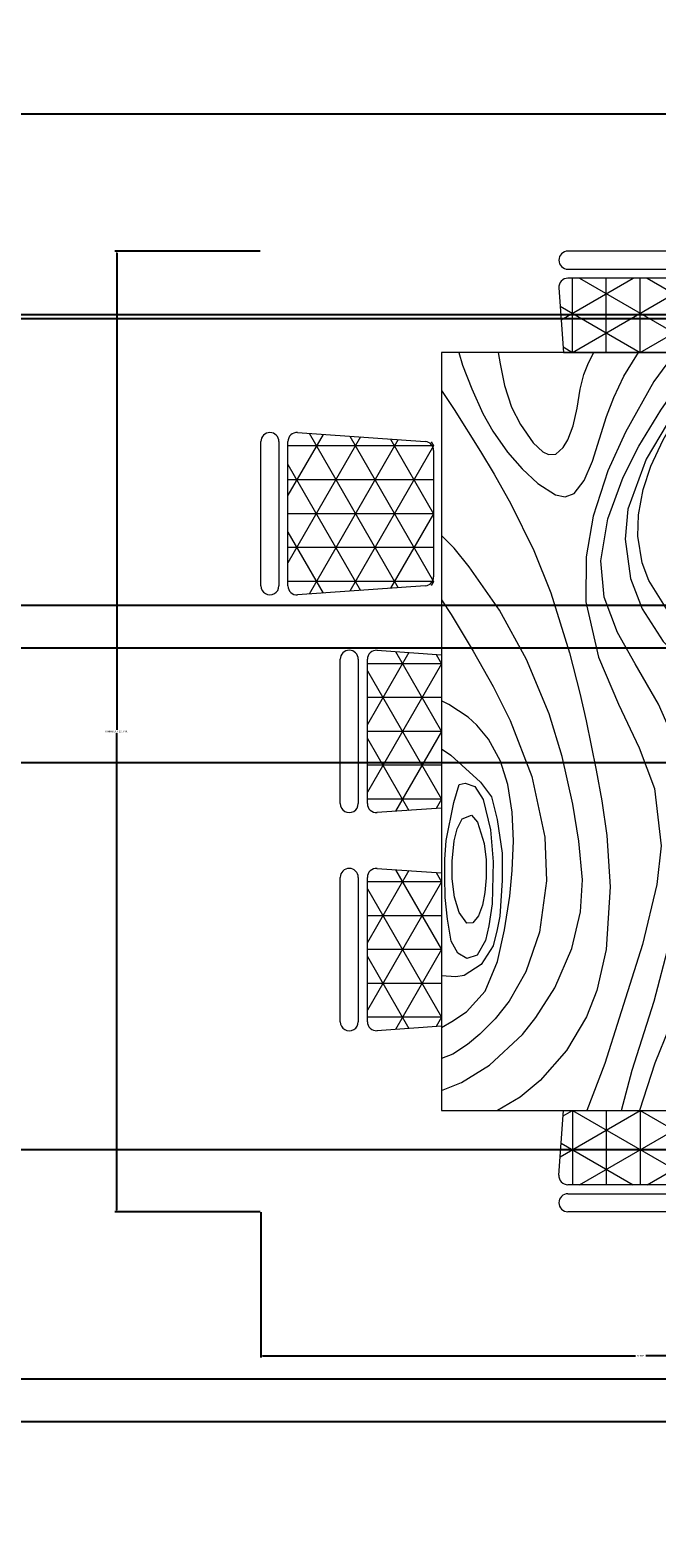
# Model space of a CAD drawing. Units: inches. Extents: x 5716 to 6907, y 12769 to 13594.
# Tile 5 of 17: x 5941 to 6007, y 13109 to 13266. Entities that reach past the tile are written whole.
import ezdxf

# ---------------------------------------------------------------- set-up
doc = ezdxf.new("R2010")
doc.units = ezdxf.units.IN
doc.layers.add('A-ANNO-DIMS', color=2, linetype='Continuous', lineweight=18)
doc.layers.add('A-FURN', color=8, linetype='Continuous', lineweight=18)
doc.styles.get("Standard").update_dxf_attribs({"font": 'arial.ttf'})
doc.dimstyles.get("Standard").update_dxf_attribs({"dimtxt": 0.18, "dimasz": 0.18, "dimexe": 0.18, "dimexo": 0.0625, "dimgap": 0.09, "dimtad": 0, "dimtih": 1, "dimtoh": 1, "dimdec": 4, "dimzin": 0, "dimdsep": 46, "dimtxsty": 'Standard', "dimcen": 0.09, "dimadec": 0, "dimazin": 0, "dimtfac": 1, "dimtdec": 4, "dimtofl": 0, "dimtmove": 0, "dimatfit": 3, "dimfxl": 1, "dimtolj": 1, "dimtzin": 0, "dimarcsym": 0})

# ---------------------------------------------------------------- blocks, each defined once
blk = doc.blocks.new('A$C405465A0')
for p, q in [((1.1305, 2.1034), (1.5301, 2.1034)), ((1.5301, 2.0534), (1.1305, 2.0534)), ((1.279, 2.0284), (1.1105, 1.9312)), ((1.4665, 2.0284), (1.1178, 1.8271)), ((1.1305, 2.0284), (1.5301, 2.0284)), ((1.1428, 1.625), (1.1428, 2.0284)), ((1.5427, 1.8271), (1.1941, 2.0284)), ((1.2365, 1.625), (1.2365, 2.0284)), ((1.3303, 1.625), (1.3303, 2.0284)), ((1.5501, 1.9312), (1.3816, 2.0284)), ((1.424, 1.625), (1.424, 2.0284)), ((1.5178, 1.625), (1.5178, 2.0284)), ((1.1304, 1.6481), (1.1055, 2.0017)), ((1.5354, 1.7231), (1.1078, 1.97)), ((1.5528, 1.97), (1.1252, 1.7231)), ((1.555, 2.0017), (1.5301, 1.6481)), ((0.9452, 1.8803), (0.5455, 1.8803)), ((2.1342, 1.8803), (1.7345, 1.8803)), ((1.5178, 1.625), (1.1157, 1.8572)), ((1.5449, 1.8572), (1.1428, 1.625)), ((0.5268, 1.6904), (0.7259, 1.8053)), ((0.5455, 1.8303), (0.9452, 1.8303)), ((0.9452, 1.8053), (0.5455, 1.8053)), ((0.5578, 1.6), (0.5578, 1.8053)), ((0.5578, 1.6), (0.9134, 1.8053)), ((0.5773, 1.8053), (0.9328, 1.6)), ((0.6516, 1.6), (0.6516, 1.8053)), ((0.7453, 1.6), (0.7453, 1.8053)), ((0.7648, 1.8053), (0.9639, 1.6904)), ((0.8391, 1.6), (0.8391, 1.8053)), ((0.9328, 1.6), (0.9328, 1.8053)), ((1.7158, 1.6904), (1.9149, 1.8053)), ((1.7345, 1.8303), (2.1342, 1.8303)), ((2.1342, 1.8053), (1.7345, 1.8053)), ((1.7468, 1.6), (1.7468, 1.8053)), ((1.7468, 1.6), (2.1024, 1.8053)), ((1.7663, 1.8053), (2.1218, 1.6)), ((1.8406, 1.6), (1.8406, 1.8053)), ((1.9343, 1.6), (1.9343, 1.8053)), ((1.9538, 1.8053), (2.1529, 1.6904)), ((2.0281, 1.6), (2.0281, 1.8053)), ((2.1218, 1.6), (2.1218, 1.8053)), ((0.5206, 1.7786), (0.5332, 1.6)), ((0.9575, 1.6), (0.9701, 1.7786)), ((1.7096, 1.7786), (1.7222, 1.6)), ((2.1465, 1.6), (2.1591, 1.7786)), ((0.5242, 1.7277), (0.7453, 1.6)), ((0.7453, 1.6), (0.9665, 1.7277)), ((1.3303, 1.625), (1.1237, 1.7443)), ((1.5369, 1.7443), (1.3303, 1.625)), ((1.7132, 1.7277), (1.9343, 1.6)), ((1.9343, 1.6), (2.1555, 1.7277)), ((1.1428, 1.625), (1.1316, 1.6315)), ((1.529, 1.6315), (1.5178, 1.625)), ((2.3803, 1.6), (0.2803, 1.6)), ((0.2803, 1.6), (0.2803, 0.5)), ((0.5321, 1.6149), (0.5578, 1.6)), ((0.5332, 1.6), (0.9575, 1.6)), ((0.7152, 1.6), (0.7236, 1.5766)), ((0.9055, 1.5469), (0.8836, 1.6)), ((0.9328, 1.6), (0.9586, 1.6149)), ((1.0212, 1.6), (1.0194, 1.5656)), ((1.1269, 1.5706), (1.1432, 1.6)), ((1.5052, 1.625), (1.1554, 1.625)), ((1.1922, 1.5507), (1.214, 1.6)), ((1.3907, 1.6), (1.3616, 1.5541)), ((1.7211, 1.6149), (1.7468, 1.6)), ((1.7222, 1.6), (2.1465, 1.6)), ((1.9386, 1.6), (1.9093, 1.5754)), ((2.1086, 1.5664), (2.17, 1.6)), ((2.1218, 1.6), (2.1476, 1.6149)), ((2.3803, 1.5967), (2.3153, 1.558)), ((2.3803, 0.5), (2.3803, 1.6)), ((0.3956, 1.553), (0.3856, 1.5163)), ((0.4356, 1.5842), (0.3956, 1.553)), ((0.5827, 1.5379), (0.4356, 1.5842)), ((0.7236, 1.5766), (0.7578, 1.4998)), ((0.9296, 1.4669), (0.9055, 1.5469)), ((1.0194, 1.5656), (1.026, 1.5003)), ((1.1178, 1.5243), (1.1269, 1.5706)), ((1.1887, 1.5196), (1.1922, 1.5507)), ((1.3616, 1.5541), (1.3027, 1.5125)), ((1.9093, 1.5754), (1.8386, 1.5427)), ((1.9962, 1.5248), (2.1086, 1.5664)), ((2.3153, 1.558), (2.1962, 1.4994)), ((0.3856, 1.5163), (0.4538, 1.4363)), ((0.4482, 1.5094), (0.4582, 1.5336)), ((0.4595, 1.4847), (0.4482, 1.5094)), ((0.4582, 1.5336), (0.5016, 1.5339)), ((0.5016, 1.5339), (0.54, 1.5204)), ((0.54, 1.5204), (0.5786, 1.5)), ((0.6365, 1.5019), (0.5827, 1.5379)), ((1.1128, 1.4699), (1.1178, 1.5243)), ((1.2089, 1.4946), (1.1887, 1.5196)), ((1.3027, 1.5125), (1.2618, 1.4976)), ((1.446, 1.5079), (1.3392, 1.4609)), ((1.5543, 1.5261), (1.446, 1.5079)), ((1.6627, 1.5271), (1.5543, 1.5261)), ((1.7679, 1.5301), (1.6627, 1.5271)), ((1.8386, 1.5427), (1.7679, 1.5301)), ((1.8488, 1.4892), (1.9962, 1.5248)), ((2.215, 1.4381), (2.3447, 1.5068)), ((2.3447, 1.5068), (2.3803, 1.5269)), ((0.4876, 1.4521), (0.4595, 1.4847)), ((0.5786, 1.5), (0.6151, 1.4744)), ((0.6151, 1.4744), (0.6557, 1.4351)), ((0.7193, 1.4377), (0.6365, 1.5019)), ((0.7578, 1.4998), (0.7752, 1.4525)), ((0.9436, 1.385), (0.9296, 1.4669)), ((1.026, 1.5003), (1.0343, 1.4559)), ((1.1133, 1.4295), (1.1128, 1.4699)), ((1.2618, 1.4976), (1.2089, 1.4946)), ((1.4396, 1.445), (1.5179, 1.4625)), ((1.5179, 1.4625), (1.717, 1.474)), ((1.717, 1.474), (1.8488, 1.4892)), ((2.1962, 1.4994), (2.0887, 1.4564)), ((0.3744, 1.3943), (0.2803, 1.458)), ((0.4538, 1.4363), (0.5034, 1.394)), ((0.5099, 1.4328), (0.4876, 1.4521)), ((0.5366, 1.4137), (0.5099, 1.4328)), ((0.6557, 1.4351), (0.6746, 1.4025)), ((0.7442, 1.4091), (0.7193, 1.4377)), ((0.7752, 1.4525), (0.7871, 1.4053)), ((1.0343, 1.4559), (1.0488, 1.3883)), ((1.1222, 1.3821), (1.1133, 1.4295)), ((1.3392, 1.4609), (1.2655, 1.4131)), ((1.3398, 1.3841), (1.4396, 1.445)), ((1.9879, 1.4268), (1.8502, 1.4019)), ((2.0887, 1.4564), (1.9879, 1.4268)), ((2.1089, 1.3912), (2.215, 1.4381)), ((0.4543, 1.3479), (0.3744, 1.3943)), ((0.5034, 1.394), (0.551, 1.3648)), ((0.5694, 1.3947), (0.5366, 1.4137)), ((0.597, 1.3823), (0.5694, 1.3947)), ((0.6281, 1.3731), (0.597, 1.3823)), ((0.674, 1.3825), (0.654, 1.3714)), ((0.6746, 1.4025), (0.674, 1.3825)), ((0.746, 1.3555), (0.7442, 1.4091)), ((0.7871, 1.4053), (0.7898, 1.3706)), ((0.9447, 1.3133), (0.9436, 1.385)), ((1.0488, 1.3883), (1.0626, 1.2943)), ((1.1508, 1.3537), (1.1222, 1.3821)), ((1.2655, 1.4131), (1.2034, 1.3712)), ((1.2659, 1.3078), (1.3398, 1.3841)), ((1.5407, 1.3902), (1.4616, 1.3726)), ((1.6315, 1.3907), (1.5407, 1.3902)), ((1.7291, 1.3922), (1.6315, 1.3907)), ((1.8502, 1.4019), (1.7291, 1.3922)), ((1.9689, 1.3731), (2.0551, 1.3789)), ((2.0551, 1.3789), (2.1089, 1.3912)), ((2.1327, 1.3477), (2.1998, 1.3905)), ((2.1998, 1.3905), (2.271, 1.4021)), ((2.271, 1.4021), (2.3264, 1.3943)), ((2.3264, 1.3943), (2.3803, 1.3943)), ((0.2803, 1.3424), (0.3226, 1.3046)), ((0.523, 1.3203), (0.4543, 1.3479)), ((0.551, 1.3648), (0.5952, 1.3458)), ((0.5952, 1.3458), (0.6524, 1.335)), ((0.654, 1.3714), (0.6281, 1.3731)), ((0.7159, 1.3352), (0.746, 1.3555)), ((0.7898, 1.3706), (0.7722, 1.3216)), ((1.2034, 1.3712), (1.1508, 1.3537)), ((1.4211, 1.3426), (1.398, 1.3071)), ((1.4616, 1.3726), (1.4211, 1.3426)), ((1.8309, 1.3257), (1.8869, 1.3472)), ((1.8869, 1.3472), (1.9689, 1.3731)), ((2.1112, 1.3052), (2.1327, 1.3477)), ((2.2336, 1.2914), (2.2346, 1.3391)), ((2.2346, 1.3391), (2.2726, 1.3593)), ((2.2726, 1.3593), (2.339, 1.3581)), ((2.339, 1.3581), (2.3803, 1.3581)), ((0.3226, 1.3046), (0.3891, 1.2586)), ((0.6007, 1.301), (0.523, 1.3203)), ((0.6623, 1.3018), (0.6007, 1.301)), ((0.6524, 1.335), (0.7159, 1.3352)), ((0.7385, 1.3018), (0.6623, 1.3018)), ((0.7722, 1.3216), (0.7385, 1.3018)), ((0.9305, 1.2479), (0.9447, 1.3133)), ((1.1689, 1.1968), (1.2659, 1.3078)), ((1.398, 1.3071), (1.412, 1.2681)), ((1.8267, 1.2783), (1.8309, 1.3257)), ((2.1264, 1.2714), (2.1112, 1.3052)), ((0.075, 1.0695), (0.19, 1.2686)), ((0.2803, 1.2622), (0.1018, 1.2748)), ((0.2803, 1.05), (0.1526, 1.2712)), ((0.2803, 1.2375), (0.2654, 1.2633)), ((0.3797, 1.2052), (0.2803, 1.2816)), ((0.2803, 0.8379), (0.2803, 1.2622)), ((0.3891, 1.2586), (0.4808, 1.2074)), ((1.0626, 1.2943), (1.06, 1.2384)), ((1.412, 1.2681), (1.4535, 1.2416)), ((1.8814, 1.2462), (1.8267, 1.2783)), ((2.171, 1.2386), (2.1264, 1.2714)), ((2.2746, 1.2504), (2.2336, 1.2914)), ((2.3803, 1.2622), (2.5588, 1.2748)), ((2.3803, 1.05), (2.508, 1.2712)), ((2.3803, 1.2375), (2.3951, 1.2633)), ((2.3803, 0.8379), (2.3803, 1.2622)), ((2.5856, 1.0695), (2.4706, 1.2686)), ((0, 1.2499), (0, 0.8502)), ((0.05, 0.8502), (0.05, 1.2499)), ((0.075, 1.2499), (0.075, 0.8502)), ((0.2803, 1.2375), (0.075, 1.2375)), ((0.075, 0.882), (0.2803, 1.2375)), ((0.2803, 0.8625), (0.075, 1.2181)), ((0.2803, 1.2498), (0.478, 1.1251)), ((0.3728, 1.1548), (0.2803, 1.2123)), ((0.8894, 1.1911), (0.9305, 1.2479)), ((1.06, 1.2384), (1.0402, 1.1815)), ((1.4535, 1.2416), (1.5203, 1.2085)), ((1.5203, 1.2085), (1.5912, 1.2143)), ((1.5912, 1.2143), (1.7027, 1.2151)), ((1.7027, 1.2151), (1.8282, 1.1987)), ((1.9819, 1.2225), (1.8814, 1.2462)), ((2.1048, 1.2108), (1.9819, 1.2225)), ((2.2593, 1.2028), (2.171, 1.2386)), ((2.3417, 1.2285), (2.2746, 1.2504)), ((2.3803, 1.226), (2.3417, 1.2285)), ((2.3803, 1.2375), (2.5856, 1.2375)), ((2.5856, 0.882), (2.3803, 1.2375)), ((2.3803, 0.8625), (2.5856, 1.2181)), ((2.5856, 1.2499), (2.5856, 0.8502)), ((2.6106, 0.8502), (2.6106, 1.2499)), ((2.6606, 1.2499), (2.6606, 0.8502)), ((0.4682, 1.1454), (0.3797, 1.2052)), ((0.4808, 1.2074), (0.5771, 1.1712)), ((0.5771, 1.1712), (0.7161, 1.1491)), ((0.8213, 1.159), (0.8894, 1.1911)), ((1.0402, 1.1815), (0.9932, 1.1252)), ((1.0809, 1.1136), (1.1689, 1.1968)), ((1.6097, 1.1755), (1.4537, 1.1662)), ((1.757, 1.1624), (1.6097, 1.1755)), ((1.8282, 1.1987), (1.9236, 1.1792)), ((1.9236, 1.1792), (2.049, 1.1552)), ((2.1888, 1.194), (2.1048, 1.2108)), ((2.2653, 1.1704), (2.1888, 1.194)), ((2.3339, 1.1841), (2.2593, 1.2028)), ((2.3396, 1.1432), (2.2653, 1.1704)), ((2.3803, 1.1754), (2.3339, 1.1841)), ((0.2803, 1.1438), (0.075, 1.1438)), ((0.2803, 1.1471), (0.3609, 1.0879)), ((0.4405, 1.1078), (0.3728, 1.1548)), ((0.5225, 1.114), (0.4682, 1.1454)), ((0.7161, 1.1491), (0.8213, 1.159)), ((1.3237, 1.1316), (1.2549, 1.1012)), ((1.4537, 1.1662), (1.3237, 1.1316)), ((1.9184, 1.131), (1.757, 1.1624)), ((2.0769, 1.0887), (1.9184, 1.131)), ((2.049, 1.1552), (2.1515, 1.1303)), ((2.1515, 1.1303), (2.2486, 1.0908)), ((2.3803, 1.126), (2.3396, 1.1432)), ((2.3803, 1.1438), (2.5856, 1.1438)), ((0.3609, 1.0879), (0.5015, 1.0099)), ((0.5402, 1.0464), (0.4405, 1.1078)), ((0.478, 1.1251), (0.576, 1.067)), ((0.5954, 1.0801), (0.5225, 1.114)), ((0.9932, 1.1252), (0.9121, 1.0739)), ((0.9908, 1.0561), (1.0809, 1.1136)), ((1.2549, 1.1012), (1.1432, 1.0368)), ((1.3755, 1.0479), (1.4887, 1.0901)), ((1.4887, 1.0901), (1.6473, 1.1088)), ((1.6473, 1.1088), (1.7544, 1.0961)), ((1.7544, 1.0961), (1.9207, 1.0564)), ((2.2686, 1.0282), (2.0769, 1.0887)), ((2.2486, 1.0908), (2.3803, 1.048)), ((0.2803, 1.05), (0.075, 1.05)), ((0.1526, 0.8289), (0.2803, 1.05)), ((0.3078, 1.029), (0.2803, 1.0458)), ((0.6261, 1.0028), (0.5402, 1.0464)), ((0.576, 1.067), (0.7146, 1.0163)), ((0.6603, 1.0585), (0.5954, 1.0801)), ((0.7308, 1.0454), (0.6603, 1.0585)), ((0.7897, 1.0439), (0.7308, 1.0454)), ((0.863, 1.056), (0.7897, 1.0439)), ((0.9121, 1.0739), (0.863, 1.056)), ((0.9069, 1.0237), (0.9908, 1.0561)), ((1.2543, 0.9907), (1.3755, 1.0479)), ((1.9207, 1.0564), (2.1244, 0.9922)), ((2.3803, 1.05), (2.5856, 1.05)), ((2.508, 0.8289), (2.3803, 1.05)), ((0.19, 0.8315), (0.075, 1.0306)), ((0.346, 1.0052), (0.3078, 1.029)), ((0.4051, 0.9771), (0.346, 1.0052)), ((0.5015, 1.0099), (0.6086, 0.961)), ((0.7415, 0.9604), (0.6261, 1.0028)), ((0.7146, 1.0163), (0.7979, 1.0084)), ((0.7979, 1.0084), (0.9069, 1.0237)), ((1.1432, 1.0368), (1.0559, 0.9876)), ((2.3803, 0.9983), (2.2686, 1.0282)), ((2.4706, 0.8315), (2.5856, 1.0306)), ((0.4579, 0.9575), (0.4051, 0.9771)), ((0.6086, 0.961), (0.7339, 0.9201)), ((0.8579, 0.9417), (0.7415, 0.9604)), ((1.0559, 0.9876), (0.958, 0.9508)), ((1.1244, 0.9348), (1.2543, 0.9907)), ((1.6187, 0.9581), (1.7607, 0.9676)), ((1.7607, 0.9676), (1.9339, 0.9563)), ((2.1244, 0.9922), (2.2495, 0.9522)), ((0.2803, 0.9563), (0.075, 0.9563)), ((0.309, 0.9074), (0.2803, 0.9224)), ((0.5195, 0.9378), (0.4579, 0.9575)), ((0.5818, 0.918), (0.5195, 0.9378)), ((0.7339, 0.9201), (0.8463, 0.9008)), ((0.958, 0.9508), (0.8579, 0.9417)), ((0.9714, 0.9002), (1.1244, 0.9348)), ((1.301, 0.9003), (1.4378, 0.9282)), ((1.4378, 0.9282), (1.5224, 0.9439)), ((1.5224, 0.9439), (1.6187, 0.9581)), ((1.9339, 0.9563), (2.0478, 0.9301)), ((2.0478, 0.9301), (2.1209, 0.9013)), ((2.2495, 0.9522), (2.3803, 0.9025)), ((2.3803, 0.9563), (2.5856, 0.9563)), ((0.342, 0.8943), (0.309, 0.9074)), ((0.3823, 0.8837), (0.342, 0.8943)), ((0.4349, 0.876), (0.3823, 0.8837)), ((0.6352, 0.8954), (0.5818, 0.918)), ((0.6712, 0.8671), (0.6352, 0.8954)), ((0.8463, 0.9008), (0.9714, 0.9002)), ((1.1125, 0.8545), (1.224, 0.8829)), ((1.224, 0.8829), (1.301, 0.9003)), ((1.6341, 0.8806), (1.5313, 0.864)), ((1.7415, 0.8904), (1.6341, 0.8806)), ((1.8296, 0.8853), (1.7415, 0.8904)), ((1.9317, 0.8609), (1.8296, 0.8853)), ((2.1209, 0.9013), (2.214, 0.8459)), ((0.2803, 0.8625), (0.075, 0.8625)), ((0.1018, 0.8253), (0.2803, 0.8379)), ((0.2654, 0.8368), (0.2803, 0.8625)), ((0.4843, 0.8652), (0.4349, 0.876)), ((0.5229, 0.85), (0.4843, 0.8652)), ((0.5441, 0.8372), (0.5229, 0.85)), ((0.5622, 0.8164), (0.5441, 0.8372)), ((0.6805, 0.8424), (0.6712, 0.8671)), ((0.675, 0.8159), (0.6805, 0.8424)), ((0.9468, 0.8025), (1.1125, 0.8545)), ((1.5313, 0.864), (1.3995, 0.834)), ((2.0406, 0.8138), (1.9317, 0.8609)), ((2.214, 0.8459), (2.297, 0.7736)), ((2.3803, 0.8625), (2.5856, 0.8625)), ((2.3951, 0.8368), (2.3803, 0.8625)), ((2.5588, 0.8253), (2.3803, 0.8379)), ((0.5562, 0.7809), (0.5634, 0.7968)), ((0.5634, 0.7968), (0.5622, 0.8164)), ((0.6434, 0.7666), (0.675, 0.8159)), ((0.8288, 0.7556), (0.9468, 0.8025)), ((1.2818, 0.7979), (1.131, 0.7357)), ((1.3995, 0.834), (1.2818, 0.7979)), ((2.1229, 0.7618), (2.0406, 0.8138)), ((0.4801, 0.7185), (0.5313, 0.7537)), ((0.5313, 0.7537), (0.5562, 0.7809)), ((0.603, 0.7231), (0.6434, 0.7666)), ((0.6995, 0.6921), (0.8288, 0.7556)), ((1.4547, 0.7504), (1.6229, 0.7863)), ((1.6229, 0.7863), (1.7436, 0.7907)), ((1.7436, 0.7907), (1.8858, 0.7711)), ((1.8858, 0.7711), (1.9957, 0.7333)), ((2.1698, 0.724), (2.1229, 0.7618)), ((2.297, 0.7736), (2.3432, 0.7176)), ((0.4317, 0.6944), (0.4801, 0.7185)), ((0.5568, 0.6828), (0.603, 0.7231)), ((1.131, 0.7357), (0.9946, 0.6604)), ((1.2995, 0.6899), (1.4547, 0.7504)), ((1.9957, 0.7333), (2.0772, 0.6873)), ((2.2541, 0.6328), (2.1698, 0.724)), ((2.3432, 0.7176), (2.3803, 0.6555)), ((0.312, 0.6622), (0.3723, 0.6742)), ((0.3723, 0.6742), (0.4317, 0.6944)), ((0.499, 0.6426), (0.5568, 0.6828)), ((0.6181, 0.6464), (0.6995, 0.6921)), ((1.2062, 0.6433), (1.2995, 0.6899)), ((1.4772, 0.6838), (1.4124, 0.6631)), ((1.554, 0.696), (1.4772, 0.6838)), ((1.6333, 0.6993), (1.554, 0.696)), ((1.7153, 0.696), (1.6333, 0.6993)), ((1.6677, 0.668), (1.7434, 0.6684)), ((1.7865, 0.6892), (1.7153, 0.696)), ((1.7434, 0.6684), (1.8417, 0.6617)), ((1.8794, 0.6748), (1.7865, 0.6892)), ((1.9674, 0.6548), (1.8794, 0.6748)), ((2.0772, 0.6873), (2.1261, 0.6491)), ((0.2803, 0.6573), (0.312, 0.6622)), ((0.4497, 0.615), (0.499, 0.6426)), ((0.5546, 0.6082), (0.6181, 0.6464)), ((0.9946, 0.6604), (0.8746, 0.5766)), ((1.1078, 0.5882), (1.2062, 0.6433)), ((1.3518, 0.6302), (1.3133, 0.5983)), ((1.4124, 0.6631), (1.3518, 0.6302)), ((1.4712, 0.6079), (1.5115, 0.6388)), ((1.5115, 0.6388), (1.5744, 0.6543)), ((1.5188, 0.6159), (1.6031, 0.6361)), ((1.5744, 0.6543), (1.6677, 0.668)), ((1.6031, 0.6361), (1.6918, 0.6436)), ((1.6918, 0.6436), (1.8075, 0.6404)), ((1.8075, 0.6404), (1.8682, 0.6312)), ((1.8417, 0.6617), (1.8785, 0.6547)), ((1.8682, 0.6312), (1.909, 0.622)), ((1.8785, 0.6547), (1.9243, 0.6434)), ((1.9243, 0.6434), (1.9761, 0.6102)), ((2.0494, 0.621), (1.9674, 0.6548)), ((2.1261, 0.6491), (2.1688, 0.6067)), ((2.3022, 0.5551), (2.2541, 0.6328)), ((0.3813, 0.5837), (0.4497, 0.615)), ((0.4385, 0.5349), (0.5546, 0.6082)), ((1.0064, 0.5273), (1.1078, 0.5882)), ((1.3133, 0.5983), (1.2908, 0.5736)), ((1.3959, 0.5264), (1.4712, 0.6079)), ((1.4736, 0.5658), (1.4828, 0.5927)), ((1.4828, 0.5927), (1.5188, 0.6159)), ((1.5621, 0.583), (1.5815, 0.6002)), ((1.5815, 0.6002), (1.641, 0.6183)), ((1.641, 0.6183), (1.6861, 0.6235)), ((1.6861, 0.6235), (1.7353, 0.624)), ((1.7353, 0.624), (1.7765, 0.6204)), ((1.7765, 0.6204), (1.811, 0.6136)), ((1.811, 0.6136), (1.8414, 0.6025)), ((1.8414, 0.6025), (1.8603, 0.5873)), ((1.8603, 0.5873), (1.8611, 0.5702)), ((1.909, 0.622), (1.9497, 0.5991)), ((1.9497, 0.5991), (1.9595, 0.5705)), ((1.9761, 0.6102), (2.006, 0.5625)), ((2.1071, 0.5697), (2.0494, 0.621)), ((2.1688, 0.6067), (2.197, 0.5721)), ((0.2803, 0.5477), (0.3159, 0.5583)), ((0.3159, 0.5583), (0.3813, 0.5837)), ((0.8746, 0.5766), (0.8225, 0.5348)), ((1.2908, 0.5736), (1.2556, 0.52)), ((1.4775, 0.5489), (1.4736, 0.5658)), ((1.5273, 0.534), (1.4775, 0.5489)), ((1.572, 0.557), (1.5621, 0.583)), ((1.5997, 0.5436), (1.572, 0.557)), ((1.6329, 0.5353), (1.5997, 0.5436)), ((1.8321, 0.5488), (1.7888, 0.5363)), ((1.8611, 0.5702), (1.8321, 0.5488)), ((1.9448, 0.5456), (1.9108, 0.5271)), ((1.9595, 0.5705), (1.9448, 0.5456)), ((2.006, 0.5625), (2.0103, 0.5395)), ((2.1338, 0.529), (2.1071, 0.5697)), ((2.197, 0.5721), (2.2242, 0.5314)), ((2.3248, 0.5), (2.3022, 0.5551)), ((0.3857, 0.5), (0.4385, 0.5349)), ((0.8225, 0.5348), (0.7878, 0.5)), ((0.9657, 0.5), (1.0064, 0.5273)), ((1.2556, 0.52), (1.2455, 0.5)), ((1.3784, 0.5), (1.3959, 0.5264)), ((1.6327, 0.513), (1.5273, 0.534)), ((1.685, 0.5094), (1.6327, 0.513)), ((1.6895, 0.5294), (1.6329, 0.5353)), ((1.7331, 0.5091), (1.685, 0.5094)), ((1.7388, 0.53), (1.6895, 0.5294)), ((1.7906, 0.5103), (1.7331, 0.5091)), ((1.7888, 0.5363), (1.7388, 0.53)), ((1.8503, 0.5169), (1.7906, 0.5103)), ((1.9108, 0.5271), (1.8503, 0.5169)), ((2.0103, 0.5395), (2.0069, 0.5)), ((2.1506, 0.5), (2.1338, 0.529)), ((2.2242, 0.5314), (2.2363, 0.5)), ((0.2803, 0.5), (2.3803, 0.5)), ((0.5126, 0.2463), (0.9147, 0.4784)), ((0.5205, 0.3591), (0.7272, 0.4784)), ((0.5285, 0.4719), (0.5397, 0.4784)), ((0.5397, 0.4784), (0.5397, 0.075)), ((0.5397, 0.4784), (0.9417, 0.2463)), ((0.5522, 0.4784), (0.9021, 0.4784)), ((0.6334, 0.4784), (0.6334, 0.075)), ((0.7272, 0.4784), (0.7272, 0.075)), ((0.7272, 0.4784), (0.9338, 0.3591)), ((0.8209, 0.4784), (0.8209, 0.075)), ((0.9147, 0.4784), (0.9147, 0.075)), ((0.9147, 0.4784), (0.9258, 0.4719)), ((1.1055, 0.3215), (1.1181, 0.5)), ((1.1091, 0.3724), (1.3303, 0.5)), ((1.1171, 0.4852), (1.1428, 0.5)), ((1.1181, 0.5), (1.5425, 0.5)), ((1.1428, 0.5), (1.1428, 0.2948)), ((1.1428, 0.5), (1.4984, 0.2948)), ((1.1622, 0.2948), (1.5178, 0.5)), ((1.2365, 0.5), (1.2365, 0.2948)), ((1.3303, 0.5), (1.3303, 0.2948)), ((1.3303, 0.5), (1.5515, 0.3724)), ((1.424, 0.5), (1.424, 0.2948)), ((1.5178, 0.5), (1.5178, 0.2948)), ((1.5178, 0.5), (1.5435, 0.4852)), ((1.5425, 0.5), (1.555, 0.3215)), ((1.7096, 0.3215), (1.7222, 0.5)), ((1.7132, 0.3724), (1.9343, 0.5)), ((1.7211, 0.4852), (1.7468, 0.5)), ((1.7222, 0.5), (2.1465, 0.5)), ((1.7468, 0.5), (1.7468, 0.2948)), ((1.7468, 0.5), (2.1024, 0.2948)), ((1.7663, 0.2948), (2.1218, 0.5)), ((1.8406, 0.5), (1.8406, 0.2948)), ((1.9343, 0.5), (1.9343, 0.2948)), ((1.9343, 0.5), (2.1555, 0.3724)), ((2.0281, 0.5), (2.0281, 0.2948)), ((2.1218, 0.5), (2.1218, 0.2948)), ((2.1218, 0.5), (2.1476, 0.4852)), ((2.1465, 0.5), (2.1591, 0.3215)), ((0.5024, 0.1018), (0.5273, 0.4553)), ((0.927, 0.4553), (0.9519, 0.1018)), ((0.5046, 0.1334), (0.9323, 0.3803)), ((0.522, 0.3803), (0.9497, 0.1334)), ((1.1118, 0.4097), (1.3109, 0.2948)), ((1.3497, 0.2948), (1.5488, 0.4097)), ((1.7158, 0.4097), (1.9149, 0.2948)), ((1.9538, 0.2948), (2.1529, 0.4097)), ((1.5301, 0.2948), (1.1305, 0.2948)), ((2.1342, 0.2948), (1.7345, 0.2948)), ((0.5147, 0.2763), (0.8634, 0.075)), ((0.591, 0.075), (0.9396, 0.2763)), ((1.1305, 0.2698), (1.5301, 0.2698)), ((1.7345, 0.2698), (2.1342, 0.2698)), ((1.5301, 0.2198), (1.1305, 0.2198)), ((2.1342, 0.2198), (1.7345, 0.2198)), ((0.5074, 0.1723), (0.6759, 0.075)), ((0.7785, 0.075), (0.9469, 0.1723)), ((0.927, 0.075), (0.5273, 0.075)), ((0.5273, 0.05), (0.927, 0.05)), ((0.927, 0), (0.5273, 0))]:
    blk.add_line(p, q)
for centre, start, end in [((1.1305, 2.0784), 90, 270), ((1.5301, 2.0784), 270, 90), ((1.1305, 2.0034), 90, 184.0274), ((1.5301, 2.0034), 355.9726, 90), ((0.5455, 1.8553), 90, 270), ((0.9452, 1.8553), 270, 90), ((1.7345, 1.8553), 90, 270), ((2.1342, 1.8553), 270, 90), ((0.5455, 1.7803), 90, 184.0274), ((0.9452, 1.7803), 355.9726, 90), ((1.7345, 1.7803), 90, 184.0274), ((2.1342, 1.7803), 355.9726, 90), ((1.1554, 1.65), 184.3987, 270), ((1.5052, 1.65), 270, 355.6013), ((0.025, 1.2499), 0, 180), ((0.1, 1.2499), 85.9726, 180), ((2.5606, 1.2499), 0, 94.0274), ((2.6356, 1.2499), 0, 180), ((0.025, 0.8502), 180, 0), ((0.1, 0.8502), 180, 274.0274), ((2.5606, 0.8502), 265.9726, 0), ((2.6356, 0.8502), 180, 0), ((0.5522, 0.4534), 90, 175.6013), ((0.9021, 0.4534), 4.3987, 90), ((1.1305, 0.3198), 175.9726, 270), ((1.5301, 0.3198), 270, 4.0274), ((1.7345, 0.3198), 175.9726, 270), ((2.1342, 0.3198), 270, 4.0274), ((1.1305, 0.2448), 90, 270), ((1.5301, 0.2448), 270, 90), ((1.7345, 0.2448), 90, 270), ((2.1342, 0.2448), 270, 90), ((0.5273, 0.1), 175.9726, 270), ((0.927, 0.1), 270, 4.0274), ((0.5273, 0.025), 90, 270), ((0.927, 0.025), 270, 90)]:
    blk.add_arc(centre, 0.025, start, end)
blk = doc.blocks.new('*D37')
at = {"layer": 'A-ANNO-DIMS', "color": 0, "lineweight": -2, "transparency": 16777216}
for p, q in [((5965.02, 13243.2), (5949.81, 13243.2)), ((5949.99, 13243.02), (5949.99, 13193.1)), ((5949.99, 13142.82), (5949.99, 13192.74)), ((5965.02, 13142.64), (5949.81, 13142.64))]:
    blk.add_line(p, q, dxfattribs=at)
at = {"layer": 'A-ANNO-DIMS', "color": 0, "transparency": 16777216}
for points in [[(5949.96, 13243.02), (5950.02, 13243.02), (5949.99, 13243.2)], [(5949.96, 13142.82), (5950.02, 13142.82), (5949.99, 13142.64)]]:
    blk.add_solid(points, dxfattribs=at)
at = {"layer": 'Defpoints', "color": 0, "transparency": 16777216}
for p in [(5965.08, 13243.2), (5949.99, 13142.64), (5965.08, 13142.64)]:
    blk.add_point(p, dxfattribs=at)
at = {"layer": 'A-ANNO-DIMS', "color": 0, "transparency": 16777216, "insert": (5949.99, 13192.92), "char_height": 0.18, "attachment_point": 5}
blk.add_mtext('\\A1;DINING SET 101 TYP.', dxfattribs=at)
blk = doc.blocks.new('*D38')
at = {"layer": 'A-ANNO-DIMS', "color": 0, "lineweight": -2, "transparency": 16777216}
for p, q in [((5965.08, 13142.58), (5965.08, 13127.37)), ((6044.58, 13142.58), (6044.58, 13127.37)), ((5965.26, 13127.55), (6004.3, 13127.55)), ((6044.4, 13127.55), (6005.36, 13127.55))]:
    blk.add_line(p, q, dxfattribs=at)
at = {"layer": 'A-ANNO-DIMS', "color": 0, "transparency": 16777216}
for points in [[(5965.26, 13127.58), (5965.26, 13127.52), (5965.08, 13127.55)], [(6044.4, 13127.58), (6044.4, 13127.52), (6044.58, 13127.55)]]:
    blk.add_solid(points, dxfattribs=at)
at = {"layer": 'Defpoints', "color": 0, "transparency": 16777216}
for p in [(5965.08, 13142.64), (6044.58, 13142.64), (6044.58, 13127.55)]:
    blk.add_point(p, dxfattribs=at)
at = {"layer": 'A-ANNO-DIMS', "color": 0, "transparency": 16777216, "insert": (6004.83, 13127.55), "char_height": 0.18, "attachment_point": 5}
blk.add_mtext('\\A1;80 TYP.', dxfattribs=at)
blk = doc.blocks.new('*D51')
at = {"layer": 'A-ANNO-DIMS', "color": 0, "lineweight": -2, "transparency": 16777216}
for p, q in [((5819.02, 13440.21), (5819.02, 13594.38)), ((5819.2, 13594.2), (6033.23, 13594.2)), ((6247.84, 13594.2), (6033.82, 13594.2)), ((6248.02, 13194.21), (6248.02, 13594.38))]:
    blk.add_line(p, q, dxfattribs=at)
at = {"layer": 'A-ANNO-DIMS', "color": 0, "transparency": 16777216}
for points in [[(5819.2, 13594.23), (5819.2, 13594.17), (5819.02, 13594.2)], [(6247.84, 13594.23), (6247.84, 13594.17), (6248.02, 13594.2)]]:
    blk.add_solid(points, dxfattribs=at)
at = {"layer": 'Defpoints', "color": 0, "transparency": 16777216}
for p in [(6248.02, 13594.2), (5819.02, 13440.15), (6248.02, 13194.15)]:
    blk.add_point(p, dxfattribs=at)
at = {"layer": 'A-ANNO-DIMS', "color": 0, "transparency": 16777216, "insert": (6033.52, 13594.2), "char_height": 0.18, "attachment_point": 5}
blk.add_mtext('\\A1;429', dxfattribs=at)
blk = doc.blocks.new('*D52')
at = {"layer": 'A-ANNO-DIMS', "color": 0, "lineweight": -2, "transparency": 16777216}
for p, q in [((6267.34, 13440.15), (5716.04, 13440.15)), ((5716.22, 13439.97), (5716.22, 13140.83)), ((5716.22, 12841.33), (5716.22, 13140.47)), ((6267.34, 12841.15), (5716.04, 12841.15))]:
    blk.add_line(p, q, dxfattribs=at)
at = {"layer": 'A-ANNO-DIMS', "color": 0, "transparency": 16777216}
for points in [[(5716.19, 13439.97), (5716.25, 13439.97), (5716.22, 13440.15)], [(5716.19, 12841.33), (5716.25, 12841.33), (5716.22, 12841.15)]]:
    blk.add_solid(points, dxfattribs=at)
at = {"layer": 'Defpoints', "color": 0, "transparency": 16777216}
for p in [(6267.41, 13440.15), (5716.22, 12841.15), (6267.41, 12841.15)]:
    blk.add_point(p, dxfattribs=at)
at = {"layer": 'A-ANNO-DIMS', "color": 0, "transparency": 16777216, "insert": (5716.22, 13140.65), "char_height": 0.18, "attachment_point": 5}
blk.add_mtext('\\A1;599', dxfattribs=at)
blk = doc.blocks.new('*D59')
at = {"layer": 'A-ANNO-DIMS', "color": 0, "lineweight": -2, "transparency": 16777216}
for p, q in [((6736.67, 13294.65), (5716.04, 13294.65)), ((5716.22, 13294.47), (5716.22, 13248.33)), ((5716.22, 13201.83), (5716.22, 13247.97)), ((6736.67, 13201.65), (5716.04, 13201.65))]:
    blk.add_line(p, q, dxfattribs=at)
at = {"layer": 'A-ANNO-DIMS', "color": 0, "transparency": 16777216}
for points in [[(5716.19, 13294.47), (5716.25, 13294.47), (5716.22, 13294.65)], [(5716.19, 13201.83), (5716.25, 13201.83), (5716.22, 13201.65)]]:
    blk.add_solid(points, dxfattribs=at)
at = {"layer": 'Defpoints', "color": 0, "transparency": 16777216}
for p in [(6736.73, 13294.65), (5716.22, 13201.65), (6736.73, 13201.65)]:
    blk.add_point(p, dxfattribs=at)
at = {"layer": 'A-ANNO-DIMS', "color": 0, "transparency": 16777216, "insert": (5716.22, 13248.15), "char_height": 0.18, "attachment_point": 5}
blk.add_mtext('\\A1;93', dxfattribs=at)
blk = doc.blocks.new('*D60')
at = {"layer": 'A-ANNO-DIMS', "color": 0, "lineweight": -2, "transparency": 16777216}
for p, q in [((6736.67, 13201.65), (5716.04, 13201.65)), ((5716.22, 13201.47), (5716.22, 13195.83)), ((5716.22, 13189.83), (5716.22, 13195.47)), ((6827.78, 13189.65), (5716.04, 13189.65))]:
    blk.add_line(p, q, dxfattribs=at)
at = {"layer": 'A-ANNO-DIMS', "color": 0, "transparency": 16777216}
for points in [[(5716.19, 13201.47), (5716.25, 13201.47), (5716.22, 13201.65)], [(5716.19, 13189.83), (5716.25, 13189.83), (5716.22, 13189.65)]]:
    blk.add_solid(points, dxfattribs=at)
at = {"layer": 'Defpoints', "color": 0, "transparency": 16777216}
for p in [(6736.73, 13201.65), (5716.22, 13189.65), (6827.84, 13189.65)]:
    blk.add_point(p, dxfattribs=at)
at = {"layer": 'A-ANNO-DIMS', "color": 0, "transparency": 16777216, "insert": (5716.22, 13195.65), "char_height": 0.18, "attachment_point": 5}
blk.add_mtext('\\A1;12', dxfattribs=at)
blk = doc.blocks.new('*D61')
at = {"layer": 'A-ANNO-DIMS', "color": 0, "lineweight": -2, "transparency": 16777216}
for p, q in [((6827.78, 13189.65), (5716.04, 13189.65)), ((5716.22, 13189.47), (5716.22, 13155.33)), ((5716.22, 13120.83), (5716.22, 13154.97)), ((6736.67, 13120.65), (5716.04, 13120.65))]:
    blk.add_line(p, q, dxfattribs=at)
at = {"layer": 'A-ANNO-DIMS', "color": 0, "transparency": 16777216}
for points in [[(5716.19, 13189.47), (5716.25, 13189.47), (5716.22, 13189.65)], [(5716.19, 13120.83), (5716.25, 13120.83), (5716.22, 13120.65)]]:
    blk.add_solid(points, dxfattribs=at)
at = {"layer": 'Defpoints', "color": 0, "transparency": 16777216}
for p in [(6827.84, 13189.65), (5716.22, 13120.65), (6736.73, 13120.65)]:
    blk.add_point(p, dxfattribs=at)
at = {"layer": 'A-ANNO-DIMS', "color": 0, "transparency": 16777216, "insert": (5716.22, 13155.15), "char_height": 0.18, "attachment_point": 5}
blk.add_mtext('\\A1;69', dxfattribs=at)
blk = doc.blocks.new('*D62')
at = {"layer": 'A-ANNO-DIMS', "color": 0, "lineweight": -2, "transparency": 16777216}
for p, q in [((6736.67, 13120.65), (5716.04, 13120.65)), ((5716.22, 13120.47), (5716.22, 13100.33)), ((5716.22, 13079.83), (5716.22, 13099.97)), ((6736.67, 13079.65), (5716.04, 13079.65))]:
    blk.add_line(p, q, dxfattribs=at)
at = {"layer": 'A-ANNO-DIMS', "color": 0, "transparency": 16777216}
for points in [[(5716.19, 13120.47), (5716.25, 13120.47), (5716.22, 13120.65)], [(5716.19, 13079.83), (5716.25, 13079.83), (5716.22, 13079.65)]]:
    blk.add_solid(points, dxfattribs=at)
at = {"layer": 'Defpoints', "color": 0, "transparency": 16777216}
for p in [(6736.73, 13120.65), (5716.22, 13079.65), (6736.73, 13079.65)]:
    blk.add_point(p, dxfattribs=at)
at = {"layer": 'A-ANNO-DIMS', "color": 0, "transparency": 16777216, "insert": (5716.22, 13100.15), "char_height": 0.18, "attachment_point": 5}
blk.add_mtext('\\A1;41', dxfattribs=at)
blk = doc.blocks.new('*D69')
at = {"layer": 'A-ANNO-DIMS', "color": 0, "lineweight": -2, "transparency": 16777216}
for p, q in [((5828.09, 13149.15), (6907.26, 13149.15)), ((6907.08, 13148.97), (6907.08, 13137.33)), ((6907.08, 13125.33), (6907.08, 13136.97)), ((5828.09, 13125.15), (6907.26, 13125.15))]:
    blk.add_line(p, q, dxfattribs=at)
at = {"layer": 'A-ANNO-DIMS', "color": 0, "transparency": 16777216}
for points in [[(6907.05, 13148.97), (6907.11, 13148.97), (6907.08, 13149.15)], [(6907.05, 13125.33), (6907.11, 13125.33), (6907.08, 13125.15)]]:
    blk.add_solid(points, dxfattribs=at)
at = {"layer": 'Defpoints', "color": 0, "transparency": 16777216}
for p in [(5828.02, 13149.15), (6907.08, 13149.15), (5828.02, 13125.15)]:
    blk.add_point(p, dxfattribs=at)
at = {"layer": 'A-ANNO-DIMS', "color": 0, "transparency": 16777216, "insert": (6907.08, 13137.15), "char_height": 0.18, "attachment_point": 5}
blk.add_mtext('\\A1;24', dxfattribs=at)
blk = doc.blocks.new('*D70')
at = {"layer": 'A-ANNO-DIMS', "color": 0, "lineweight": -2, "transparency": 16777216}
for p, q in [((5828.09, 13236.15), (6907.26, 13236.15)), ((6907.08, 13235.97), (6907.08, 13221.33)), ((6907.08, 13206.33), (6907.08, 13220.97)), ((5828.09, 13206.15), (6907.26, 13206.15))]:
    blk.add_line(p, q, dxfattribs=at)
at = {"layer": 'A-ANNO-DIMS', "color": 0, "transparency": 16777216}
for points in [[(6907.05, 13235.97), (6907.11, 13235.97), (6907.08, 13236.15)], [(6907.05, 13206.33), (6907.11, 13206.33), (6907.08, 13206.15)]]:
    blk.add_solid(points, dxfattribs=at)
at = {"layer": 'Defpoints', "color": 0, "transparency": 16777216}
for p in [(5828.02, 13236.15), (6907.08, 13236.15), (5828.02, 13206.15)]:
    blk.add_point(p, dxfattribs=at)
at = {"layer": 'A-ANNO-DIMS', "color": 0, "transparency": 16777216, "insert": (6907.08, 13221.15), "char_height": 0.18, "attachment_point": 5}
blk.add_mtext('\\A1;30', dxfattribs=at)
blk = doc.blocks.new('*D76')
at = {"layer": 'A-ANNO-DIMS', "color": 0, "lineweight": -2, "transparency": 16777216}
for p, q in [((5830.73, 13257.56), (6907.26, 13257.56)), ((6907.08, 13257.38), (6907.08, 13247.24)), ((6907.08, 13236.74), (6907.08, 13246.88)), ((5830.73, 13236.56), (6907.26, 13236.56))]:
    blk.add_line(p, q, dxfattribs=at)
at = {"layer": 'A-ANNO-DIMS', "color": 0, "transparency": 16777216}
for points in [[(6907.05, 13257.38), (6907.11, 13257.38), (6907.08, 13257.56)], [(6907.05, 13236.74), (6907.11, 13236.74), (6907.08, 13236.56)]]:
    blk.add_solid(points, dxfattribs=at)
at = {"layer": 'Defpoints', "color": 0, "transparency": 16777216}
for p in [(5830.67, 13257.56), (5830.67, 13236.56), (6907.08, 13236.56)]:
    blk.add_point(p, dxfattribs=at)
at = {"layer": 'A-ANNO-DIMS', "color": 0, "transparency": 16777216, "insert": (6907.08, 13247.06), "char_height": 0.18, "attachment_point": 5}
blk.add_mtext('\\A1;21', dxfattribs=at)

msp = doc.modelspace()

# ---------------------------------------------------------------- block references
at = {"layer": 'A-FURN', "xscale": 37.79737452882042, "yscale": 37.79737452882042, "zscale": 37.79737452882042, "rotation": 270}
msp.add_blockref('A$C405465A0', (5965.08, 13243.2), dxfattribs=at)

# ---------------------------------------------------------------- dimensions: what is measured, and where the dimension line sits
at = {"layer": 'A-ANNO-DIMS'}
dim = msp.add_linear_dim(base=(6248.02, 13594.2), p1=(5819.02, 13440.15), p2=(6248.02, 13194.15), dimstyle='Standard', override={"dimdec": 0, "dimlfac": 1, "dimrnd": 0, "dimzin": 0, "dimdsep": 46, "dimlunit": 2}, dxfattribs=at)
dim.commit()
dim.dimension.update_dxf_attribs({"geometry": '*D51', "text_midpoint": (6033.52, 13594.2)})
for base, p1, p2, picture, middle in [((5716.22, 12841.15), (6267.41, 13440.15), (6267.41, 12841.15), '*D52', (5716.22, 13140.65)), ((5716.22, 13201.65), (6736.73, 13294.65), (6736.73, 13201.65), '*D59', (5716.22, 13248.15)), ((6907.08, 13236.56), (5830.67, 13257.56), (5830.67, 13236.56), '*D76', (6907.08, 13247.06)), ((6907.08, 13236.15), (5828.02, 13206.15), (5828.02, 13236.15), '*D70', (6907.08, 13221.15)), ((5716.22, 13189.65), (6736.73, 13201.65), (6827.84, 13189.65), '*D60', (5716.22, 13195.65)), ((5716.22, 13120.65), (6827.84, 13189.65), (6736.73, 13120.65), '*D61', (5716.22, 13155.15)), ((6907.08, 13149.15), (5828.02, 13125.15), (5828.02, 13149.15), '*D69', (6907.08, 13137.15)), ((5716.22, 13079.65), (6736.73, 13120.65), (6736.73, 13079.65), '*D62', (5716.22, 13100.15))]:
    dim = msp.add_linear_dim(base=base, p1=p1, p2=p2, angle=90, dimstyle='Standard', override={"dimdec": 0, "dimlfac": 1, "dimrnd": 0, "dimzin": 0, "dimdsep": 46, "dimlunit": 2}, dxfattribs=at)
    dim.commit()
    dim.dimension.update_dxf_attribs({"geometry": picture, "text_midpoint": middle})
dim = msp.add_linear_dim(base=(5949.99, 13142.64), p1=(5965.08, 13243.2), p2=(5965.08, 13142.64), angle=270, text='DINING SET <> TYP.', dimstyle='Standard', override={"dimdec": 0, "dimlfac": 1, "dimrnd": 0, "dimzin": 0, "dimdsep": 46, "dimlunit": 2}, dxfattribs=at)
dim.commit()
dim.dimension.update_dxf_attribs({"geometry": '*D37', "text_midpoint": (5949.99, 13192.92)})
dim = msp.add_linear_dim(base=(6044.5823, 13127.5543), p1=(5965.0776, 13142.6388), p2=(6044.5823, 13142.6388), text='<> TYP.', dimstyle='Standard', override={"dimdec": 0, "dimlfac": 1, "dimrnd": 0, "dimzin": 0, "dimdsep": 46, "dimlunit": 2}, dxfattribs=at)
dim.commit()
dim.dimension.update_dxf_attribs({"geometry": '*D38', "text_midpoint": (6004.8299, 13127.5543)})

doc.saveas('drawing.dxf')
